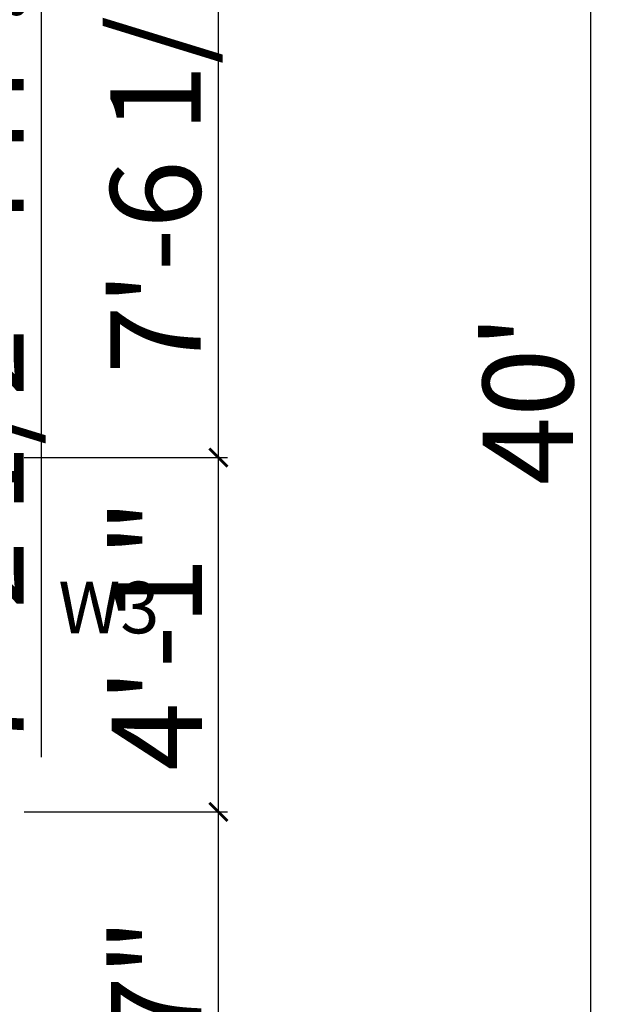
# Model space of a CAD drawing. Units: inches. Extents: x 1763 to 2368, y 1500 to 2097.
# Tile 16 of 24: x 2189 to 2269, y 1720 to 1856. Entities that reach past the tile are written whole.
import ezdxf

# ---------------------------------------------------------------- set-up
doc = ezdxf.new("R2010")
doc.units = ezdxf.units.IN
doc.layers.add('A-ANNO-DIMS', color=2, linetype='Continuous', lineweight=18)
doc.layers.add('A-ANNO-TEXT', color=7, linetype='Continuous', lineweight=18)
doc.styles.get("Standard").update_dxf_attribs({"font": 'arial.ttf'})
doc.dimstyles.new('ISO-25', dxfattribs={"dimtxt": 12.5, "dimasz": 2.5, "dimexe": 1.25, "dimexo": 0.625, "dimtad": 1, "dimdec": 0, "dimlunit": 4, "dimtxsty": 'Standard', "dimblk": 'ARCHTICK', "dimcen": 2.5, "dimclrd": 3, "dimclrt": 4, "dimadec": 0, "dimazin": 0, "dimtfac": 1, "dimtdec": 0, "dimtmove": 0, "dimatfit": 3, "dimfxl": 1, "dimarcsym": 0})

# ---------------------------------------------------------------- blocks, each defined once
blk = doc.blocks.new('_ArchTick')
at = {"color": 0, "linetype": 'ByBlock', "const_width": 0.15}
blk.add_lwpolyline([(-0.5, -0.5), (0.5, 0.5)], dxfattribs=at)
blk = doc.blocks.new('*D22')
at = {"layer": 'A-ANNO-DIMS', "color": 0, "lineweight": -2, "transparency": 16777216}
for p, q in [((2189.72, 2043.27), (2269.32, 2043.27)), ((2268.07, 2043.27), (2268.07, 1563.27)), ((2189.72, 1563.27), (2269.32, 1563.27))]:
    blk.add_line(p, q, dxfattribs=at)
at = {"layer": 'Defpoints', "color": 0, "transparency": 16777216}
for p in [(2189.09, 2043.27), (2189.09, 1563.27), (2268.07, 1563.27)]:
    blk.add_point(p, dxfattribs=at)
at = {"layer": 'A-ANNO-DIMS', "color": 0, "lineweight": -2, "transparency": 16777216, "xscale": 2.5, "yscale": 2.5, "zscale": 2.5}
for p, rotation in [((2268.07, 2043.27), 90), ((2268.07, 1563.27), 270)]:
    blk.add_blockref('_ArchTick', p, dxfattribs=dict(at, rotation=rotation))
at = {"layer": 'A-ANNO-DIMS', "color": 0, "transparency": 16777216, "insert": (2261.06, 1803.27), "char_height": 12.5, "attachment_point": 5, "rotation": 90}
blk.add_mtext("40'", dxfattribs=at)
blk = doc.blocks.new('*D24')
at = {"layer": 'A-ANNO-DIMS', "color": 0, "lineweight": -2, "transparency": 16777216}
for p, q in [((2179.32, 1949.35), (2193.33, 1949.35)), ((2179.32, 1862.76), (2193.33, 1862.76))]:
    blk.add_line(p, q, dxfattribs=at)
at = {"layer": 'A-ANNO-DIMS', "color": 3, "lineweight": -2, "transparency": 16777216}
for p, q in [((2192.08, 1949.35), (2192.08, 1862.76)), ((2192.08, 1862.76), (2192.08, 1753.79))]:
    blk.add_line(p, q, dxfattribs=at)
at = {"layer": 'Defpoints', "color": 0, "transparency": 16777216}
for p in [(2178.7, 1949.35), (2178.7, 1862.76), (2192.08, 1862.76)]:
    blk.add_point(p, dxfattribs=at)
at = {"layer": 'A-ANNO-DIMS', "color": 3, "lineweight": -2, "transparency": 16777216, "xscale": 2.5, "yscale": 2.5, "zscale": 2.5}
for p, rotation in [((2192.08, 1949.35), 90), ((2192.08, 1862.76), 270)]:
    blk.add_blockref('_ArchTick', p, dxfattribs=dict(at, rotation=rotation))
at = {"layer": 'A-ANNO-DIMS', "color": 4, "transparency": 16777216, "insert": (2184.99, 1807.02), "char_height": 12.5, "attachment_point": 5, "rotation": 90}
blk.add_mtext('7\'-2 1/2" TYP.', dxfattribs=at)
blk = doc.blocks.new('*D52')
at = {"layer": 'A-ANNO-DIMS', "color": 0, "lineweight": -2, "transparency": 16777216}
for p, q in [((2189.72, 1746.22), (2217.84, 1746.22)), ((2180.72, 1679.27), (2217.84, 1679.27))]:
    blk.add_line(p, q, dxfattribs=at)
at = {"layer": 'A-ANNO-DIMS', "color": 3, "lineweight": -2, "transparency": 16777216}
blk.add_line((2216.59, 1679.27), (2216.59, 1746.22), dxfattribs=at)
at = {"layer": 'Defpoints', "color": 0, "transparency": 16777216}
for p in [(2189.09, 1746.22), (2216.59, 1746.22), (2180.09, 1679.27)]:
    blk.add_point(p, dxfattribs=at)
at = {"layer": 'A-ANNO-DIMS', "color": 3, "lineweight": -2, "transparency": 16777216, "xscale": 2.5, "yscale": 2.5, "zscale": 2.5}
for p, rotation in [((2216.59, 1746.22), 90), ((2216.59, 1679.27), 270)]:
    blk.add_blockref('_ArchTick', p, dxfattribs=dict(at, rotation=rotation))
at = {"layer": 'A-ANNO-DIMS', "color": 4, "transparency": 16777216, "insert": (2209.61, 1712.75), "char_height": 12.5, "attachment_point": 5, "rotation": 90}
blk.add_mtext('5\'-7"', dxfattribs=at)
blk = doc.blocks.new('*D53')
at = {"layer": 'A-ANNO-DIMS', "color": 0, "lineweight": -2, "transparency": 16777216}
for p, q in [((2189.72, 1795.26), (2217.84, 1795.26)), ((2189.72, 1746.22), (2217.84, 1746.22))]:
    blk.add_line(p, q, dxfattribs=at)
at = {"layer": 'A-ANNO-DIMS', "color": 3, "lineweight": -2, "transparency": 16777216}
blk.add_line((2216.59, 1746.22), (2216.59, 1795.26), dxfattribs=at)
at = {"layer": 'Defpoints', "color": 0, "transparency": 16777216}
for p in [(2189.09, 1795.26), (2216.59, 1795.26), (2189.09, 1746.22)]:
    blk.add_point(p, dxfattribs=at)
at = {"layer": 'A-ANNO-DIMS', "color": 3, "lineweight": -2, "transparency": 16777216, "xscale": 2.5, "yscale": 2.5, "zscale": 2.5}
for p, rotation in [((2216.59, 1795.26), 90), ((2216.59, 1746.22), 270)]:
    blk.add_blockref('_ArchTick', p, dxfattribs=dict(at, rotation=rotation))
at = {"layer": 'A-ANNO-DIMS', "color": 4, "transparency": 16777216, "insert": (2209.69, 1770.74), "char_height": 12.5, "attachment_point": 5, "rotation": 90}
blk.add_mtext('4\'-1"', dxfattribs=at)
blk = doc.blocks.new('*D54')
at = {"layer": 'A-ANNO-DIMS', "color": 0, "lineweight": -2, "transparency": 16777216}
for p, q in [((2189.72, 1885.52), (2217.84, 1885.52)), ((2189.72, 1795.26), (2217.84, 1795.26))]:
    blk.add_line(p, q, dxfattribs=at)
at = {"layer": 'A-ANNO-DIMS', "color": 3, "lineweight": -2, "transparency": 16777216}
blk.add_line((2216.59, 1795.26), (2216.59, 1885.52), dxfattribs=at)
at = {"layer": 'Defpoints', "color": 0, "transparency": 16777216}
for p in [(2189.09, 1885.52), (2216.59, 1885.52), (2189.09, 1795.26)]:
    blk.add_point(p, dxfattribs=at)
at = {"layer": 'A-ANNO-DIMS', "color": 3, "lineweight": -2, "transparency": 16777216, "xscale": 2.5, "yscale": 2.5, "zscale": 2.5}
for p, rotation in [((2216.59, 1885.52), 90), ((2216.59, 1795.26), 270)]:
    blk.add_blockref('_ArchTick', p, dxfattribs=dict(at, rotation=rotation))
at = {"layer": 'A-ANNO-DIMS', "color": 4, "transparency": 16777216, "insert": (2209.5, 1840.39), "char_height": 12.5, "attachment_point": 5, "rotation": 90}
blk.add_mtext('7\'-6 1/2"', dxfattribs=at)

msp = doc.modelspace()

# ---------------------------------------------------------------- texts
at = {"layer": 'A-ANNO-TEXT'}
msp.add_text('W3', height=7.155, dxfattribs=at).set_placement((2194.44, 1770.94))

# ---------------------------------------------------------------- dimensions: what is measured, and where the dimension line sits
at = {"layer": 'A-ANNO-DIMS'}
for base, p1, p2, override, picture, middle in [((2268.07, 1563.27), (2189.09, 2043.27), (2189.09, 1563.27), {"dimclrd": 0, "dimclre": 0, "dimclrt": 0}, '*D22', (2261.06, 1803.27)), ((2216.59, 1885.52), (2189.09, 1795.26), (2189.09, 1885.52), {"dimdec": 1, "dimlfac": 1, "dimrnd": 0, "dimzin": 1, "dimdsep": 46, "dimlunit": 4, "dimfrac": 2}, '*D54', (2209.5, 1840.39)), ((2216.59, 1795.26), (2189.09, 1746.22), (2189.09, 1795.26), {"dimdec": 1, "dimlfac": 1, "dimrnd": 0, "dimzin": 1, "dimdsep": 46, "dimlunit": 4, "dimfrac": 2}, '*D53', (2209.69, 1770.74)), ((2216.5918, 1746.2191), (2180.0918, 1679.2727), (2189.0918, 1746.2191), {"dimdec": 1, "dimlfac": 1, "dimrnd": 0, "dimzin": 1, "dimdsep": 46, "dimlunit": 4, "dimfrac": 2}, '*D52', (2209.6102, 1712.7459))]:
    dim = msp.add_linear_dim(base=base, p1=p1, p2=p2, angle=90, dimstyle='ISO-25', override=override, dxfattribs=at)
    dim.commit()
    dim.dimension.update_dxf_attribs({"geometry": picture, "text_midpoint": middle})
dim = msp.add_linear_dim(base=(2192.08, 1862.76), p1=(2178.7, 1949.35), p2=(2178.7, 1862.76), angle=270, text='<> TYP.', dimstyle='ISO-25', override={"dimdec": 1, "dimlfac": 1, "dimrnd": 0, "dimzin": 1, "dimdsep": 46, "dimlunit": 4, "dimfrac": 2}, dxfattribs=at)
dim.commit()
dim.dimension.update_dxf_attribs({"geometry": '*D24', "text_midpoint": (2184.99, 1807.02)})

doc.saveas('drawing.dxf')
